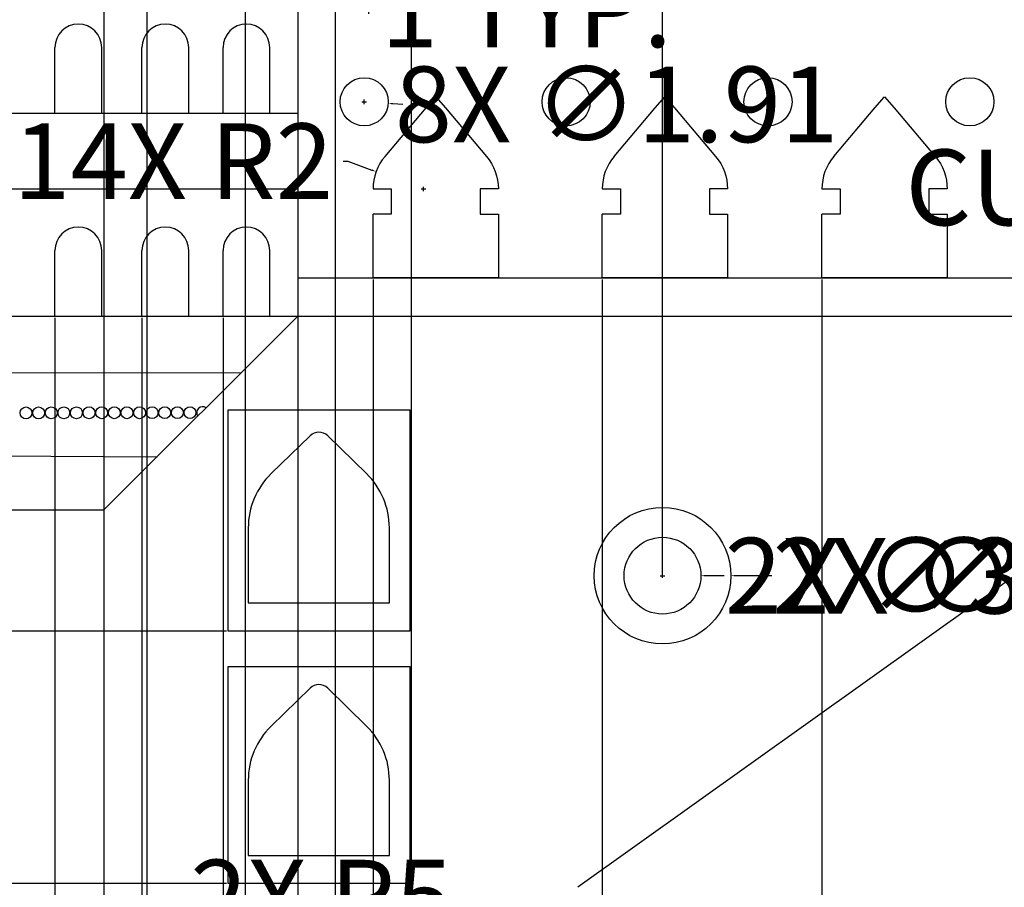
# Model space of a CAD drawing. Units: inches. Extents: x 168 to 318, y 152 to 314.
# Tile 3 of 7: x 201 to 240, y 183 to 218. Entities that reach past the tile are written whole.
import ezdxf

# ---------------------------------------------------------------- set-up
doc = ezdxf.new("R2010")
doc.units = ezdxf.units.IN
doc.header["$MEASUREMENT"] = 0
doc.layers.add('A-ANNO-DIMS', color=2, linetype='Continuous', lineweight=18)
doc.layers.add('A-ELEV', color=7, linetype='Continuous', lineweight=25)
doc.styles.get("Standard").update_dxf_attribs({"font": 'arial.ttf'})
doc.dimstyles.get("Standard").update_dxf_attribs({"dimtxt": 3, "dimasz": 0.18, "dimexe": 0.18, "dimexo": 0.0625, "dimgap": 0.09, "dimtad": 0, "dimtih": 1, "dimtoh": 1, "dimdec": 1, "dimzin": 0, "dimdsep": 46, "dimlunit": 3, "dimtxsty": 'Standard', "dimcen": 0.09, "dimadec": 0, "dimazin": 0, "dimtfac": 1, "dimtdec": 1, "dimtofl": 0, "dimtmove": 0, "dimatfit": 3, "dimfxl": 1, "dimtolj": 1, "dimtzin": 0, "dimarcsym": 0})

# ---------------------------------------------------------------- blocks, each defined once
blk = doc.blocks.new('ARCH-BALCONY-SM')
for p, q in [((0, 0), (0, 2.603)), ((1.853, 0), (1.853, 2.603))]:
    blk.add_line(p, q)
blk.add_arc((0.926, 2.603), 0.926, 0, 180)
blk = doc.blocks.new('ARCH-CUSPED-PANEL')
for p, q in [((2.1, 6.738), (2.482, 7.168)), ((2.482, 7.168), (2.864, 6.738)), ((0.472, 4.813), (2.1, 6.738)), ((2.864, 6.738), (4.491, 4.813)), ((0, 3.522), (0.2, 3.522)), ((0, 3.522), (0, 3.522)), ((0.2, 3.522), (0.719, 3.522)), ((0.719, 3.522), (0.719, 2.522)), ((4.764, 3.522), (4.244, 3.522)), ((4.244, 3.522), (4.244, 2.522)), ((4.964, 3.522), (4.764, 3.522)), ((0.719, 2.522), (0, 2.522)), ((4.244, 2.522), (4.964, 2.522))]:
    blk.add_line(p, q)
blk.add_lwpolyline([(4.491, 4.813, -0.177277), (4.964, 3.522)], format="xyb")
blk.add_lwpolyline([(4.964, 2.522), (4.964, 0), (0, 0), (0, 2.522)])
blk.add_arc((2, 3.522), 2, 139.7888, 180)
blk = doc.blocks.new('NICHE-ARCHED')
for p, q in [((0.908, 5.124), (2.451, 6.627)), ((3.149, 6.626), (4.687, 5.124)), ((0, 2.975), (0, 0)), ((5.592, 0), (5.592, 2.977)), ((0, 0), (5.592, 0))]:
    blk.add_line(p, q)
for centre, radius, start, end in [((2.8, 6.268), 0.5, 45.6844, 134.2257), ((3, 2.975), 3, 134.2257, 180), ((2.592, 2.977), 3, 0, 45.6844)]:
    blk.add_arc(centre, radius, start, end)
blk = doc.blocks.new('*D15')
at = {"layer": 'A-ANNO-DIMS', "color": 0, "lineweight": -2, "ltscale": 0.2, "transparency": 16777216}
for p, q in [((214.946, 220.875), (215.434, 220.875)), ((215.254, 220.875), (215.254, 221.055)), ((215.254, 221.055), (215.434, 221.055)), ((215.254, 218.586), (215.254, 220.695)), ((214.946, 218.406), (215.434, 218.406))]:
    blk.add_line(p, q, dxfattribs=at)
at = {"layer": 'A-ANNO-DIMS', "color": 0, "ltscale": 0.2, "transparency": 16777216}
for points in [[(215.224, 220.695), (215.284, 220.695), (215.254, 220.875)], [(215.224, 218.586), (215.284, 218.586), (215.254, 218.406)]]:
    blk.add_solid(points, dxfattribs=at)
at = {"layer": 'Defpoints', "color": 0, "ltscale": 0.2, "transparency": 16777216}
for p in [(214.883, 220.875), (215.254, 220.875), (214.883, 218.406)]:
    blk.add_point(p, dxfattribs=at)
at = {"layer": 'A-ANNO-DIMS', "color": 0, "ltscale": 0.2, "transparency": 16777216, "insert": (244.753, 221.055), "char_height": 3, "attachment_point": 5}
blk.add_mtext('\\A1;PENDANT ORNAMENT 2 TYP.', dxfattribs=at)
blk = doc.blocks.new('*D16')
at = {"layer": 'A-ANNO-DIMS', "color": 0, "lineweight": -2, "ltscale": 0.2, "transparency": 16777216}
for p, q in [((213.573, 218.343), (213.573, 217.855)), ((214.883, 218.343), (214.883, 217.855)), ((213.753, 218.035), (214.703, 218.035)), ((214.883, 218.035), (215.063, 218.035))]:
    blk.add_line(p, q, dxfattribs=at)
at = {"layer": 'A-ANNO-DIMS', "color": 0, "ltscale": 0.2, "transparency": 16777216}
for points in [[(213.753, 218.065), (213.753, 218.005), (213.573, 218.035)], [(214.703, 218.065), (214.703, 218.005), (214.883, 218.035)]]:
    blk.add_solid(points, dxfattribs=at)
at = {"layer": 'Defpoints', "color": 0, "ltscale": 0.2, "transparency": 16777216}
for p in [(213.573, 218.406), (214.883, 218.406), (214.883, 218.035)]:
    blk.add_point(p, dxfattribs=at)
at = {"layer": 'A-ANNO-DIMS', "color": 0, "ltscale": 0.2, "transparency": 16777216, "insert": (221.148, 218.035), "char_height": 3, "attachment_point": 5}
blk.add_mtext('\\A1;1 TYP.', dxfattribs=at)
blk = doc.blocks.new('*D23')
at = {"layer": 'A-ANNO-DIMS', "color": 0, "lineweight": -2, "ltscale": 0.2, "transparency": 16777216}
for p, q in [((261.882, 214.562), (263.075, 214.562)), ((262.895, 214.382), (262.895, 212.619)), ((262.895, 207.574), (262.895, 209.337)), ((261.882, 207.394), (263.075, 207.394))]:
    blk.add_line(p, q, dxfattribs=at)
at = {"layer": 'A-ANNO-DIMS', "color": 0, "ltscale": 0.2, "transparency": 16777216}
for points in [[(262.865, 214.382), (262.925, 214.382), (262.895, 214.562)], [(262.865, 207.574), (262.925, 207.574), (262.895, 207.394)]]:
    blk.add_solid(points, dxfattribs=at)
at = {"layer": 'Defpoints', "color": 0, "ltscale": 0.2, "transparency": 16777216}
for p in [(261.82, 214.562), (262.895, 214.562), (261.82, 207.394)]:
    blk.add_point(p, dxfattribs=at)
at = {"layer": 'A-ANNO-DIMS', "color": 0, "ltscale": 0.2, "transparency": 16777216, "insert": (262.895, 210.978), "char_height": 3, "attachment_point": 5}
blk.add_mtext('\\A1;CUSPED ARCH PANEL 7 TYP.', dxfattribs=at)
blk = doc.blocks.new('*D29')
at = {"layer": 'A-ANNO-DIMS', "color": 0, "lineweight": -2, "ltscale": 0.2, "transparency": 16777216}
for p, q in [((184.724, 242.139), (184.724, 154.215)), ((299.445, 242.139), (299.445, 154.215)), ((184.904, 154.395), (235.924, 154.395)), ((299.265, 154.395), (248.245, 154.395))]:
    blk.add_line(p, q, dxfattribs=at)
at = {"layer": 'A-ANNO-DIMS', "color": 0, "ltscale": 0.2, "transparency": 16777216}
for points in [[(184.904, 154.425), (184.904, 154.365), (184.724, 154.395)], [(299.265, 154.425), (299.265, 154.365), (299.445, 154.395)]]:
    blk.add_solid(points, dxfattribs=at)
at = {"layer": 'Defpoints', "color": 0, "ltscale": 0.2, "transparency": 16777216}
for p in [(184.724, 242.201), (299.445, 242.201), (299.445, 154.395)]:
    blk.add_point(p, dxfattribs=at)
at = {"layer": 'A-ANNO-DIMS', "color": 0, "ltscale": 0.2, "transparency": 16777216, "insert": (242.084, 154.395), "char_height": 3, "attachment_point": 5}
blk.add_mtext('\\A1;114.72', dxfattribs=at)
blk = doc.blocks.new('*D57')
at = {"layer": 'A-ANNO-DIMS', "color": 0, "lineweight": -2, "ltscale": 0.2, "transparency": 16777216}
for p, q in [((226.54, 195.647), (226.54, 312.411)), ((226.72, 312.231), (236.931, 312.231)), ((257.449, 312.231), (247.238, 312.231)), ((257.629, 195.647), (257.629, 312.411))]:
    blk.add_line(p, q, dxfattribs=at)
at = {"layer": 'A-ANNO-DIMS', "color": 0, "ltscale": 0.2, "transparency": 16777216}
for points in [[(226.72, 312.261), (226.72, 312.201), (226.54, 312.231)], [(257.449, 312.261), (257.449, 312.201), (257.629, 312.231)]]:
    blk.add_solid(points, dxfattribs=at)
at = {"layer": 'Defpoints', "color": 0, "ltscale": 0.2, "transparency": 16777216}
for p in [(257.629, 312.231), (226.54, 195.584), (257.629, 195.584)]:
    blk.add_point(p, dxfattribs=at)
at = {"layer": 'A-ANNO-DIMS', "color": 0, "ltscale": 0.2, "transparency": 16777216, "insert": (242.084, 312.231), "char_height": 3, "attachment_point": 5}
blk.add_mtext('\\A1;31.09', dxfattribs=at)
blk = doc.blocks.new('*D61')
at = {"layer": 'A-ANNO-DIMS', "color": 0, "lineweight": -2, "ltscale": 0.2, "transparency": 16777216}
for p, q in [((209.262, 183.379), (176.701, 183.379)), ((176.881, 183.199), (176.881, 179.852)), ((176.881, 173.262), (176.881, 176.609)), ((209.262, 173.082), (176.701, 173.082))]:
    blk.add_line(p, q, dxfattribs=at)
at = {"layer": 'A-ANNO-DIMS', "color": 0, "ltscale": 0.2, "transparency": 16777216}
for points in [[(176.851, 183.199), (176.911, 183.199), (176.881, 183.379)], [(176.851, 173.262), (176.911, 173.262), (176.881, 173.082)]]:
    blk.add_solid(points, dxfattribs=at)
at = {"layer": 'Defpoints', "color": 0, "ltscale": 0.2, "transparency": 16777216}
for p in [(176.881, 183.379), (209.325, 183.379), (209.325, 173.082)]:
    blk.add_point(p, dxfattribs=at)
at = {"layer": 'A-ANNO-DIMS', "color": 0, "ltscale": 0.2, "transparency": 16777216, "insert": (176.881, 178.231), "char_height": 3, "attachment_point": 5}
blk.add_mtext('\\A1;10.296', dxfattribs=at)
blk = doc.blocks.new('*D62')
at = {"layer": 'A-ANNO-DIMS', "color": 0, "lineweight": -2, "ltscale": 0.2, "transparency": 16777216}
for p, q in [((209.262, 193.388), (176.701, 193.388)), ((176.881, 193.208), (176.881, 190.005)), ((176.881, 183.559), (176.881, 186.762)), ((209.262, 183.379), (176.701, 183.379))]:
    blk.add_line(p, q, dxfattribs=at)
at = {"layer": 'A-ANNO-DIMS', "color": 0, "ltscale": 0.2, "transparency": 16777216}
for points in [[(176.851, 193.208), (176.911, 193.208), (176.881, 193.388)], [(176.851, 183.559), (176.911, 183.559), (176.881, 183.379)]]:
    blk.add_solid(points, dxfattribs=at)
at = {"layer": 'Defpoints', "color": 0, "ltscale": 0.2, "transparency": 16777216}
for p in [(176.881, 193.388), (209.325, 193.388), (209.325, 183.379)]:
    blk.add_point(p, dxfattribs=at)
at = {"layer": 'A-ANNO-DIMS', "color": 0, "ltscale": 0.2, "transparency": 16777216, "insert": (176.881, 188.383), "char_height": 3, "attachment_point": 5}
blk.add_mtext('\\A1;10.01', dxfattribs=at)
blk = doc.blocks.new('*D70')
at = {"layer": 'A-ANNO-DIMS', "color": 0, "lineweight": -2, "ltscale": 0.2, "transparency": 16777216}
for p, q in [((190.252, 205.813), (190.252, 154.215)), ((194.576, 205.813), (194.576, 154.215)), ((190.432, 154.395), (194.396, 154.395)), ((194.576, 154.395), (194.756, 154.395))]:
    blk.add_line(p, q, dxfattribs=at)
at = {"layer": 'A-ANNO-DIMS', "color": 0, "ltscale": 0.2, "transparency": 16777216}
for points in [[(190.432, 154.425), (190.432, 154.365), (190.252, 154.395)], [(194.396, 154.425), (194.396, 154.365), (194.576, 154.395)]]:
    blk.add_solid(points, dxfattribs=at)
at = {"layer": 'Defpoints', "color": 0, "ltscale": 0.2, "transparency": 16777216}
for p in [(190.252, 205.875), (194.576, 205.875), (194.576, 154.395)]:
    blk.add_point(p, dxfattribs=at)
at = {"layer": 'A-ANNO-DIMS', "color": 0, "ltscale": 0.2, "transparency": 16777216, "insert": (199.968, 154.395), "char_height": 3, "attachment_point": 5}
blk.add_mtext('\\A1;4.323', dxfattribs=at)
blk = doc.blocks.new('*D71')
at = {"layer": 'A-ANNO-DIMS', "color": 0, "lineweight": -2, "ltscale": 0.2, "transparency": 16777216}
for p, q in [((194.576, 205.813), (194.576, 154.215)), ((198.404, 205.813), (198.404, 154.215)), ((194.756, 154.395), (198.224, 154.395)), ((198.404, 154.395), (198.584, 154.395))]:
    blk.add_line(p, q, dxfattribs=at)
at = {"layer": 'A-ANNO-DIMS', "color": 0, "ltscale": 0.2, "transparency": 16777216}
for points in [[(194.756, 154.425), (194.756, 154.365), (194.576, 154.395)], [(198.224, 154.425), (198.224, 154.365), (198.404, 154.395)]]:
    blk.add_solid(points, dxfattribs=at)
at = {"layer": 'Defpoints', "color": 0, "ltscale": 0.2, "transparency": 16777216}
for p in [(194.576, 205.875), (198.404, 205.875), (198.404, 154.395)]:
    blk.add_point(p, dxfattribs=at)
at = {"layer": 'A-ANNO-DIMS', "color": 0, "ltscale": 0.2, "transparency": 16777216, "insert": (203.738, 154.395), "char_height": 3, "attachment_point": 5}
blk.add_mtext('\\A1;3.829', dxfattribs=at)
blk = doc.blocks.new('*D72')
at = {"layer": 'A-ANNO-DIMS', "color": 0, "lineweight": -2, "ltscale": 0.2, "transparency": 16777216}
for p, q in [((198.404, 205.813), (198.404, 154.215)), ((202.463, 205.813), (202.463, 154.215)), ((198.584, 154.395), (202.283, 154.395)), ((202.463, 154.395), (202.643, 154.395))]:
    blk.add_line(p, q, dxfattribs=at)
at = {"layer": 'A-ANNO-DIMS', "color": 0, "ltscale": 0.2, "transparency": 16777216}
for points in [[(198.584, 154.425), (198.584, 154.365), (198.404, 154.395)], [(202.283, 154.425), (202.283, 154.365), (202.463, 154.395)]]:
    blk.add_solid(points, dxfattribs=at)
at = {"layer": 'Defpoints', "color": 0, "ltscale": 0.2, "transparency": 16777216}
for p in [(198.404, 205.875), (202.463, 205.875), (202.463, 154.395)]:
    blk.add_point(p, dxfattribs=at)
at = {"layer": 'A-ANNO-DIMS', "color": 0, "ltscale": 0.2, "transparency": 16777216, "insert": (207.858, 154.395), "char_height": 3, "attachment_point": 5}
blk.add_mtext('\\A1;4.058', dxfattribs=at)
blk = doc.blocks.new('*D73')
at = {"layer": 'A-ANNO-DIMS', "color": 0, "lineweight": -2, "ltscale": 0.2, "transparency": 16777216}
for p, q in [((202.463, 205.813), (202.463, 154.215)), ((205.91, 205.813), (205.91, 154.215)), ((202.643, 154.395), (205.73, 154.395)), ((205.91, 154.395), (206.09, 154.395))]:
    blk.add_line(p, q, dxfattribs=at)
at = {"layer": 'A-ANNO-DIMS', "color": 0, "ltscale": 0.2, "transparency": 16777216}
for points in [[(202.643, 154.425), (202.643, 154.365), (202.463, 154.395)], [(205.73, 154.425), (205.73, 154.365), (205.91, 154.395)]]:
    blk.add_solid(points, dxfattribs=at)
at = {"layer": 'Defpoints', "color": 0, "ltscale": 0.2, "transparency": 16777216}
for p in [(202.463, 205.875), (205.91, 205.875), (205.91, 154.395)]:
    blk.add_point(p, dxfattribs=at)
at = {"layer": 'A-ANNO-DIMS', "color": 0, "ltscale": 0.2, "transparency": 16777216, "insert": (211.24, 154.395), "char_height": 3, "attachment_point": 5}
blk.add_mtext('\\A1;3.447', dxfattribs=at)
blk = doc.blocks.new('*D74')
at = {"layer": 'A-ANNO-DIMS', "color": 0, "lineweight": -2, "ltscale": 0.2, "transparency": 16777216}
for p, q in [((205.91, 205.813), (205.91, 154.215)), ((209.123, 205.813), (209.123, 154.215)), ((206.09, 154.395), (208.943, 154.395)), ((209.123, 154.395), (209.303, 154.395))]:
    blk.add_line(p, q, dxfattribs=at)
at = {"layer": 'A-ANNO-DIMS', "color": 0, "ltscale": 0.2, "transparency": 16777216}
for points in [[(206.09, 154.425), (206.09, 154.365), (205.91, 154.395)], [(208.943, 154.425), (208.943, 154.365), (209.123, 154.395)]]:
    blk.add_solid(points, dxfattribs=at)
at = {"layer": 'Defpoints', "color": 0, "ltscale": 0.2, "transparency": 16777216}
for p in [(205.91, 205.875), (209.123, 205.875), (209.123, 154.395)]:
    blk.add_point(p, dxfattribs=at)
at = {"layer": 'A-ANNO-DIMS', "color": 0, "ltscale": 0.2, "transparency": 16777216, "insert": (214.453, 154.395), "char_height": 3, "attachment_point": 5}
blk.add_mtext('\\A1;3.213', dxfattribs=at)
blk = doc.blocks.new('*D84')
at = {"layer": 'A-ANNO-DIMS', "color": 0, "lineweight": -2, "ltscale": 0.2, "transparency": 16777216}
for p, q in [((206.099, 227.876), (206.099, 154.215)), ((204.404, 227.113), (204.404, 154.215)), ((204.584, 154.395), (205.919, 154.395)), ((206.099, 154.395), (206.279, 154.395))]:
    blk.add_line(p, q, dxfattribs=at)
at = {"layer": 'A-ANNO-DIMS', "color": 0, "ltscale": 0.2, "transparency": 16777216}
for points in [[(204.584, 154.425), (204.584, 154.365), (204.404, 154.395)], [(205.919, 154.425), (205.919, 154.365), (206.099, 154.395)]]:
    blk.add_solid(points, dxfattribs=at)
at = {"layer": 'Defpoints', "color": 0, "ltscale": 0.2, "transparency": 16777216}
for p in [(206.099, 227.938), (204.404, 227.175), (206.099, 154.395)]:
    blk.add_point(p, dxfattribs=at)
at = {"layer": 'A-ANNO-DIMS', "color": 0, "ltscale": 0.2, "transparency": 16777216, "insert": (211.283, 154.395), "char_height": 3, "attachment_point": 5}
blk.add_mtext('\\A1;1.694', dxfattribs=at)
blk = doc.blocks.new('*D85')
at = {"layer": 'A-ANNO-DIMS', "color": 0, "lineweight": -2, "ltscale": 0.2, "transparency": 16777216}
for p, q in [((206.099, 227.876), (206.099, 154.215)), ((209.999, 227.876), (209.999, 154.215)), ((206.279, 154.395), (209.819, 154.395)), ((209.999, 154.395), (210.179, 154.395))]:
    blk.add_line(p, q, dxfattribs=at)
at = {"layer": 'A-ANNO-DIMS', "color": 0, "ltscale": 0.2, "transparency": 16777216}
for points in [[(206.279, 154.425), (206.279, 154.365), (206.099, 154.395)], [(209.819, 154.425), (209.819, 154.365), (209.999, 154.395)]]:
    blk.add_solid(points, dxfattribs=at)
at = {"layer": 'Defpoints', "color": 0, "ltscale": 0.2, "transparency": 16777216}
for p in [(206.099, 227.938), (209.999, 227.938), (209.999, 154.395)]:
    blk.add_point(p, dxfattribs=at)
at = {"layer": 'A-ANNO-DIMS', "color": 0, "ltscale": 0.2, "transparency": 16777216, "insert": (213.002, 154.395), "char_height": 3, "attachment_point": 5}
blk.add_mtext('\\A1;3.9', dxfattribs=at)
blk = doc.blocks.new('*D86')
at = {"layer": 'A-ANNO-DIMS', "color": 0, "lineweight": -2, "ltscale": 0.2, "transparency": 16777216}
for p, q in [((212.084, 220.813), (212.084, 154.215)), ((213.573, 220.813), (213.573, 154.215)), ((212.264, 154.395), (213.393, 154.395)), ((213.573, 154.395), (213.753, 154.395))]:
    blk.add_line(p, q, dxfattribs=at)
at = {"layer": 'A-ANNO-DIMS', "color": 0, "ltscale": 0.2, "transparency": 16777216}
for points in [[(212.264, 154.425), (212.264, 154.365), (212.084, 154.395)], [(213.393, 154.425), (213.393, 154.365), (213.573, 154.395)]]:
    blk.add_solid(points, dxfattribs=at)
at = {"layer": 'Defpoints', "color": 0, "ltscale": 0.2, "transparency": 16777216}
for p in [(212.084, 220.875), (213.573, 220.875), (213.573, 154.395)]:
    blk.add_point(p, dxfattribs=at)
at = {"layer": 'A-ANNO-DIMS', "color": 0, "ltscale": 0.2, "transparency": 16777216, "insert": (217.601, 154.395), "char_height": 3, "attachment_point": 5}
blk.add_mtext('\\A1;1.49', dxfattribs=at)
blk = doc.blocks.new('*D87')
at = {"layer": 'A-ANNO-DIMS', "color": 0, "lineweight": -2, "ltscale": 0.2, "transparency": 16777216}
for p, q in [((213.573, 220.813), (213.573, 154.215)), ((216.573, 220.813), (216.573, 154.215)), ((213.753, 154.395), (214.001, 154.395)), ((216.393, 154.395), (216.145, 154.395))]:
    blk.add_line(p, q, dxfattribs=at)
at = {"layer": 'A-ANNO-DIMS', "color": 0, "ltscale": 0.2, "transparency": 16777216}
for points in [[(213.753, 154.425), (213.753, 154.365), (213.573, 154.395)], [(216.393, 154.425), (216.393, 154.365), (216.573, 154.395)]]:
    blk.add_solid(points, dxfattribs=at)
at = {"layer": 'Defpoints', "color": 0, "ltscale": 0.2, "transparency": 16777216}
for p in [(213.573, 220.875), (216.573, 220.875), (216.573, 154.395)]:
    blk.add_point(p, dxfattribs=at)
at = {"layer": 'A-ANNO-DIMS', "color": 0, "ltscale": 0.2, "transparency": 16777216, "insert": (215.073, 154.395), "char_height": 3, "attachment_point": 5}
blk.add_mtext('\\A1;3', dxfattribs=at)
blk = doc.blocks.new('*D88')
at = {"layer": 'A-ANNO-DIMS', "color": 0, "lineweight": -2, "ltscale": 0.2, "transparency": 16777216}
for p, q in [((212.084, 207.331), (212.084, 154.215)), ((215.07, 207.331), (215.07, 154.215)), ((212.264, 154.395), (214.89, 154.395)), ((215.07, 154.395), (215.25, 154.395))]:
    blk.add_line(p, q, dxfattribs=at)
at = {"layer": 'A-ANNO-DIMS', "color": 0, "ltscale": 0.2, "transparency": 16777216}
for points in [[(212.264, 154.425), (212.264, 154.365), (212.084, 154.395)], [(214.89, 154.425), (214.89, 154.365), (215.07, 154.395)]]:
    blk.add_solid(points, dxfattribs=at)
at = {"layer": 'Defpoints', "color": 0, "ltscale": 0.2, "transparency": 16777216}
for p in [(212.084, 207.394), (215.07, 207.394), (215.07, 154.395)]:
    blk.add_point(p, dxfattribs=at)
at = {"layer": 'A-ANNO-DIMS', "color": 0, "ltscale": 0.2, "transparency": 16777216, "insert": (220.438, 154.395), "char_height": 3, "attachment_point": 5}
blk.add_mtext('\\A1;2.985', dxfattribs=at)
blk = doc.blocks.new('*D89')
at = {"layer": 'A-ANNO-DIMS', "color": 0, "lineweight": -2, "ltscale": 0.2, "transparency": 16777216}
for p, q in [((215.07, 207.331), (215.07, 154.215)), ((224.151, 207.331), (224.151, 154.215)), ((215.25, 154.395), (223.971, 154.395)), ((224.151, 154.395), (224.331, 154.395))]:
    blk.add_line(p, q, dxfattribs=at)
at = {"layer": 'A-ANNO-DIMS', "color": 0, "ltscale": 0.2, "transparency": 16777216}
for points in [[(215.25, 154.425), (215.25, 154.365), (215.07, 154.395)], [(223.971, 154.425), (223.971, 154.365), (224.151, 154.395)]]:
    blk.add_solid(points, dxfattribs=at)
at = {"layer": 'Defpoints', "color": 0, "ltscale": 0.2, "transparency": 16777216}
for p in [(215.07, 207.394), (224.151, 207.394), (224.151, 154.395)]:
    blk.add_point(p, dxfattribs=at)
at = {"layer": 'A-ANNO-DIMS', "color": 0, "ltscale": 0.2, "transparency": 16777216, "insert": (229.193, 154.395), "char_height": 3, "attachment_point": 5}
blk.add_mtext('\\A1;9.081', dxfattribs=at)
blk = doc.blocks.new('*D90')
at = {"layer": 'A-ANNO-DIMS', "color": 0, "lineweight": -2, "ltscale": 0.2, "transparency": 16777216}
for p, q in [((224.151, 207.331), (224.151, 154.215)), ((232.855, 207.331), (232.855, 154.215)), ((224.331, 154.395), (232.675, 154.395)), ((232.855, 154.395), (233.035, 154.395))]:
    blk.add_line(p, q, dxfattribs=at)
at = {"layer": 'A-ANNO-DIMS', "color": 0, "ltscale": 0.2, "transparency": 16777216}
for points in [[(224.331, 154.425), (224.331, 154.365), (224.151, 154.395)], [(232.675, 154.425), (232.675, 154.365), (232.855, 154.395)]]:
    blk.add_solid(points, dxfattribs=at)
at = {"layer": 'Defpoints', "color": 0, "ltscale": 0.2, "transparency": 16777216}
for p in [(224.151, 207.394), (232.855, 207.394), (232.855, 154.395)]:
    blk.add_point(p, dxfattribs=at)
at = {"layer": 'A-ANNO-DIMS', "color": 0, "ltscale": 0.2, "transparency": 16777216, "insert": (238.2, 154.395), "char_height": 3, "attachment_point": 5}
blk.add_mtext('\\A1;8.705', dxfattribs=at)
blk = doc.blocks.new('*D91')
at = {"layer": 'A-ANNO-DIMS', "color": 0, "lineweight": -2, "ltscale": 0.2, "transparency": 16777216}
for p, q in [((232.855, 207.331), (232.855, 154.215)), ((240.855, 207.331), (240.855, 154.215)), ((233.035, 154.395), (235.777, 154.395)), ((240.675, 154.395), (237.934, 154.395))]:
    blk.add_line(p, q, dxfattribs=at)
at = {"layer": 'A-ANNO-DIMS', "color": 0, "ltscale": 0.2, "transparency": 16777216}
for points in [[(233.035, 154.425), (233.035, 154.365), (232.855, 154.395)], [(240.675, 154.425), (240.675, 154.365), (240.855, 154.395)]]:
    blk.add_solid(points, dxfattribs=at)
at = {"layer": 'Defpoints', "color": 0, "ltscale": 0.2, "transparency": 16777216}
for p in [(232.855, 207.394), (240.855, 207.394), (240.855, 154.395)]:
    blk.add_point(p, dxfattribs=at)
at = {"layer": 'A-ANNO-DIMS', "color": 0, "ltscale": 0.2, "transparency": 16777216, "insert": (236.855, 154.395), "char_height": 3, "attachment_point": 5}
blk.add_mtext('\\A1;8', dxfattribs=at)
blk = doc.blocks.new('*D97')
at = {"layer": 'A-ANNO-DIMS', "color": 0, "lineweight": -2, "ltscale": 0.2, "transparency": 16777216}
for p, q in [((218.791, 182.822), (218.971, 182.822)), ((218.971, 182.822), (221.479, 181.532)), ((225.994, 179.161), (226.174, 179.161)), ((226.084, 179.071), (226.084, 179.251))]:
    blk.add_line(p, q, dxfattribs=at)
at = {"layer": 'A-ANNO-DIMS', "color": 0, "ltscale": 0.2, "transparency": 16777216}
blk.add_solid([(221.492, 181.558), (221.465, 181.505), (221.639, 181.449)], dxfattribs=at)
at = {"layer": 'Defpoints', "color": 0, "ltscale": 0.2, "transparency": 16777216}
for p in [(221.639, 181.449), (226.084, 179.161)]:
    blk.add_point(p, dxfattribs=at)
at = {"layer": 'A-ANNO-DIMS', "color": 0, "ltscale": 0.2, "transparency": 16777216, "insert": (213.023, 182.822), "char_height": 3, "attachment_point": 5}
blk.add_mtext('\\A1;2X R5', dxfattribs=at)
blk = doc.blocks.new('*D98')
at = {"layer": 'A-ANNO-DIMS', "color": 0, "lineweight": -2, "ltscale": 0.2, "transparency": 16777216}
for p, q in [((226.45, 195.584), (226.63, 195.584)), ((226.54, 195.494), (226.54, 195.674)), ((230.871, 195.584), (229.427, 195.584))]:
    blk.add_line(p, q, dxfattribs=at)
at = {"layer": 'A-ANNO-DIMS', "color": 0, "ltscale": 0.2, "transparency": 16777216}
blk.add_solid([(229.427, 195.614), (229.427, 195.554), (229.247, 195.584)], dxfattribs=at)
at = {"layer": 'Defpoints', "color": 0, "ltscale": 0.2, "transparency": 16777216}
for p in [(223.834, 195.585), (229.247, 195.584)]:
    blk.add_point(p, dxfattribs=at)
at = {"layer": 'A-ANNO-DIMS', "color": 0, "ltscale": 0.2, "transparency": 16777216, "insert": (240.824, 195.584), "char_height": 3, "attachment_point": 5}
blk.add_mtext('\\A1;2X ∅5.413', dxfattribs=at)
blk = doc.blocks.new('*D99')
at = {"layer": 'A-ANNO-DIMS', "color": 0, "lineweight": -2, "ltscale": 0.2, "transparency": 16777216}
for p, q in [((226.45, 195.584), (226.63, 195.584)), ((226.54, 195.494), (226.54, 195.674)), ((228.977, 195.584), (228.243, 195.584))]:
    blk.add_line(p, q, dxfattribs=at)
at = {"layer": 'A-ANNO-DIMS', "color": 0, "ltscale": 0.2, "transparency": 16777216}
blk.add_solid([(228.243, 195.614), (228.243, 195.554), (228.063, 195.584)], dxfattribs=at)
at = {"layer": 'Defpoints', "color": 0, "ltscale": 0.2, "transparency": 16777216}
for p in [(225.017, 195.585), (228.063, 195.584)]:
    blk.add_point(p, dxfattribs=at)
at = {"layer": 'A-ANNO-DIMS', "color": 0, "ltscale": 0.2, "transparency": 16777216, "insert": (238.928, 195.584), "char_height": 3, "attachment_point": 5}
blk.add_mtext('\\A1;2X ∅3.046', dxfattribs=at)
blk = doc.blocks.new('*D101')
at = {"layer": 'A-ANNO-DIMS', "color": 0, "lineweight": -2, "ltscale": 0.2, "transparency": 16777216}
for p, q in [((213.884, 212.015), (214.064, 212.015)), ((214.064, 212.015), (215.022, 211.665)), ((216.98, 210.916), (217.16, 210.916)), ((217.07, 210.826), (217.07, 211.006))]:
    blk.add_line(p, q, dxfattribs=at)
at = {"layer": 'A-ANNO-DIMS', "color": 0, "ltscale": 0.2, "transparency": 16777216}
blk.add_solid([(215.033, 211.693), (215.012, 211.637), (215.191, 211.603)], dxfattribs=at)
at = {"layer": 'Defpoints', "color": 0, "ltscale": 0.2, "transparency": 16777216}
for p in [(215.191, 211.603), (217.07, 210.916)]:
    blk.add_point(p, dxfattribs=at)
at = {"layer": 'A-ANNO-DIMS', "color": 0, "ltscale": 0.2, "transparency": 16777216, "insert": (207.144, 212.015), "char_height": 3, "attachment_point": 5}
blk.add_mtext('\\A1;14X R2', dxfattribs=at)
blk = doc.blocks.new('*D102')
at = {"layer": 'A-ANNO-DIMS', "color": 0, "lineweight": -2, "ltscale": 0.2, "transparency": 16777216}
for p, q in [((214.629, 214.372), (214.809, 214.372)), ((214.719, 214.282), (214.719, 214.462)), ((216.243, 214.27), (215.851, 214.296))]:
    blk.add_line(p, q, dxfattribs=at)
at = {"layer": 'A-ANNO-DIMS', "color": 0, "ltscale": 0.2, "transparency": 16777216}
blk.add_solid([(215.853, 214.326), (215.849, 214.266), (215.671, 214.308)], dxfattribs=at)
at = {"layer": 'Defpoints', "color": 0, "ltscale": 0.2, "transparency": 16777216}
for p in [(213.766, 214.435), (215.671, 214.308)]:
    blk.add_point(p, dxfattribs=at)
at = {"layer": 'A-ANNO-DIMS', "color": 0, "ltscale": 0.2, "transparency": 16777216, "insert": (224.717, 214.27), "char_height": 3, "attachment_point": 5}
blk.add_mtext('\\A1;8X ∅1.91', dxfattribs=at)

msp = doc.modelspace()

# ---------------------------------------------------------------- linework, layer by layer
at = {"layer": 'A-ELEV'}
for p, q in [((212.0845, 220.8755), (212.0845, 205.8755)), ((184.7244, 213.9241), (212.0845, 213.9241)), ((184.7244, 210.9241), (212.0845, 210.9241)), ((212.0845, 207.3935), (272.0845, 207.3935)), ((184.7244, 205.8755), (212.0845, 205.8755)), ((204.4044, 198.1954), (212.0845, 205.8755)), ((186.9522, 203.6477), (209.8404, 203.6314)), ((190.2158, 200.3841), (206.511, 200.302)), ((192.4044, 198.1954), (204.4044, 198.1954)), ((204.4044, 198.1954), (204.4044, 162.1954)), ((239.1785, 194.6573), (241.7939, 196.5252)), ((239.1785, 194.6573), (223.1785, 183.2299))]:
    msp.add_line(p, q, dxfattribs=at)
at = {"layer": 'A-ELEV', "ltscale": 0.2}
msp.add_line((212.0845, 205.8755), (272.0845, 205.8755), dxfattribs=at)
at = {"layer": 'A-ELEV'}
for points in [[(209.3248, 202.1566), (216.5216, 202.1566), (216.5216, 193.3878), (209.3248, 193.3878)], [(209.3248, 191.9874), (216.5216, 191.9874), (216.5216, 183.3788), (209.3248, 183.3788)]]:
    msp.add_lwpolyline(points, close=True, dxfattribs=at)
for centre, radius in [((214.7185, 214.3715), 0.9548), ((222.7185, 214.3715), 0.9548), ((230.7185, 214.3715), 0.9548), ((238.7185, 214.3715), 0.9548), ((201.3149, 202.0383), 0.2354), ((201.8149, 202.039), 0.2354), ((202.3149, 202.0397), 0.2354), ((202.8149, 202.0404), 0.2354), ((203.3149, 202.0412), 0.2354), ((203.8149, 202.0419), 0.2354), ((204.3149, 202.0426), 0.2354), ((204.8149, 202.0433), 0.2354), ((205.3149, 202.044), 0.2354), ((205.8149, 202.0447), 0.2354), ((206.3149, 202.0455), 0.2354), ((206.8149, 202.0462), 0.2354), ((207.3149, 202.0469), 0.2354), ((207.8149, 202.0476), 0.2354), ((226.5403, 195.5844), 2.7067), ((226.5403, 195.5844), 1.5229)]:
    msp.add_circle(centre, radius, dxfattribs=at)
msp.add_arc((208.3149, 202.0483), 0.2354, 54.95912, 215.04088, dxfattribs=at)

# ---------------------------------------------------------------- block references
for name, p in [('ARCH-BALCONY-SM', (202.4627, 213.9237)), ('ARCH-BALCONY-SM', (205.9096, 213.9237)), ('ARCH-BALCONY-SM', (209.1229, 213.9237)), ('ARCH-CUSPED-PANEL', (215.07, 207.394)), ('ARCH-CUSPED-PANEL', (224.151, 207.394)), ('ARCH-CUSPED-PANEL', (232.8558, 207.394)), ('ARCH-BALCONY-SM', (202.4627, 205.875)), ('ARCH-BALCONY-SM', (205.9096, 205.875)), ('ARCH-BALCONY-SM', (209.1229, 205.875)), ('NICHE-ARCHED', (210.123, 194.5059)), ('NICHE-ARCHED', (210.123, 184.4969))]:
    msp.add_blockref(name, p, dxfattribs=at)

# ---------------------------------------------------------------- dimensions: what is measured, and where the dimension line sits
at = {"layer": 'A-ANNO-DIMS', "ltscale": 0.2}
for base, p1, p2, override, picture, middle in [((257.6286, 312.2308), (226.5403, 195.5844), (257.6286, 195.5844), {"dimdec": 2, "dimlfac": 1, "dimrnd": 0, "dimzin": 0, "dimdsep": 46, "dimlunit": 2}, '*D57', (242.0845, 312.2308)), ((299.4446, 154.3954), (184.7244, 242.2013), (299.4446, 242.2013), {"dimdec": 2, "dimlfac": 1, "dimrnd": 0, "dimzin": 0, "dimdsep": 46, "dimlunit": 2}, '*D29', (242.0845, 154.3954)), ((206.0986, 154.3954), (204.4044, 227.1751), (206.0986, 227.9381), {"dimdec": 3, "dimlfac": 1, "dimrnd": 0, "dimzin": 0, "dimdsep": 46, "dimlunit": 2}, '*D84', (211.283, 154.3954)), ((209.9986, 154.3954), (206.0986, 227.9381), (209.9986, 227.9381), {"dimdec": 1, "dimlfac": 1, "dimrnd": 0, "dimzin": 0, "dimdsep": 46, "dimlunit": 2}, '*D85', (213.0015, 154.3954)), ((213.5729, 154.3954), (212.0845, 220.8755), (213.5729, 220.8755), {"dimdec": 2, "dimlfac": 1, "dimrnd": 0, "dimzin": 0, "dimdsep": 46, "dimlunit": 2}, '*D86', (217.601, 154.3954)), ((216.5729, 154.3954), (213.5729, 220.8755), (216.5729, 220.8755), {"dimdec": 0, "dimlfac": 1, "dimrnd": 0, "dimzin": 0, "dimdsep": 46, "dimlunit": 2}, '*D87', (215.0729, 154.3954)), ((215.0696, 154.3954), (212.0845, 207.3935), (215.0696, 207.3935), {"dimdec": 3, "dimlfac": 1, "dimrnd": 0, "dimzin": 0, "dimdsep": 46, "dimlunit": 2}, '*D88', (220.4382, 154.3954)), ((224.1506, 154.3954), (215.0696, 207.3935), (224.1506, 207.3935), {"dimdec": 3, "dimlfac": 1, "dimrnd": 0, "dimzin": 0, "dimdsep": 46, "dimlunit": 2}, '*D89', (229.1928, 154.3954)), ((232.8554, 154.3954), (224.1506, 207.3935), (232.8554, 207.3935), {"dimdec": 3, "dimlfac": 1, "dimrnd": 0, "dimzin": 0, "dimdsep": 46, "dimlunit": 2}, '*D90', (238.2004, 154.3954)), ((240.8554, 154.3954), (232.8554, 207.3935), (240.8554, 207.3935), {"dimdec": 0, "dimlfac": 1, "dimrnd": 0, "dimzin": 0, "dimdsep": 46, "dimlunit": 2}, '*D91', (236.8554, 154.3954)), ((194.5757, 154.3954), (190.2524, 205.8755), (194.5757, 205.8755), {"dimdec": 3, "dimlfac": 1, "dimrnd": 0, "dimzin": 0, "dimdsep": 46, "dimlunit": 2}, '*D70', (199.9678, 154.3954)), ((198.4044, 154.3954), (194.5757, 205.8755), (198.4044, 205.8755), {"dimdec": 3, "dimlfac": 1, "dimrnd": 0, "dimzin": 0, "dimdsep": 46, "dimlunit": 2}, '*D71', (203.7382, 154.3954)), ((202.4627, 154.3954), (198.4044, 205.8755), (202.4627, 205.8755), {"dimdec": 3, "dimlfac": 1, "dimrnd": 0, "dimzin": 0, "dimdsep": 46, "dimlunit": 2}, '*D72', (207.8578, 154.3954)), ((205.9096, 154.3954), (202.4627, 205.8755), (205.9096, 205.8755), {"dimdec": 3, "dimlfac": 1, "dimrnd": 0, "dimzin": 0, "dimdsep": 46, "dimlunit": 2}, '*D73', (211.2403, 154.3954)), ((209.1228, 154.3954), (205.9096, 205.8755), (209.1228, 205.8755), {"dimdec": 3, "dimlfac": 1, "dimrnd": 0, "dimzin": 0, "dimdsep": 46, "dimlunit": 2}, '*D74', (214.4535, 154.3954))]:
    dim = msp.add_linear_dim(base=base, p1=p1, p2=p2, dimstyle='Standard', override=override, dxfattribs=at)
    dim.commit()
    dim.dimension.update_dxf_attribs({"geometry": picture, "text_midpoint": middle})
for base, p1, p2, text, picture, middle in [((215.2539, 220.8755), (214.8834, 218.4056), (214.8834, 220.8755), 'PENDANT ORNAMENT <> TYP.', '*D15', (244.7534, 221.0555)), ((262.8949, 214.5622), (261.8196, 207.3935), (261.8196, 214.5622), 'CUSPED ARCH PANEL <> TYP.', '*D23', (262.8949, 210.9778))]:
    dim = msp.add_linear_dim(base=base, p1=p1, p2=p2, angle=90, text=text, dimstyle='Standard', override={"dimdec": 0, "dimrnd": 0, "dimzin": 0, "dimlunit": 2}, dxfattribs=at)
    dim.commit()
    dim.dimension.update_dxf_attribs({"geometry": picture, "text_midpoint": middle})
dim = msp.add_linear_dim(base=(214.8834, 218.0352), p1=(213.5729, 218.4056), p2=(214.8834, 218.4056), text='<> TYP.', dimstyle='Standard', override={"dimdec": 0, "dimrnd": 0, "dimzin": 0, "dimlunit": 2}, dxfattribs=at)
dim.commit()
dim.dimension.update_dxf_attribs({"geometry": '*D16', "text_midpoint": (221.1483, 218.0352)})
for p1, p2, text, override, picture, middle in [((213.7659, 214.4352), (215.6712, 214.3079), '8X <>', {"dimdec": 2, "dimlfac": 1, "dimrnd": 0, "dimzin": 0, "dimdsep": 46, "dimlunit": 2}, '*D102', (216.2428, 214.2697)), ((223.8336, 195.5848), (229.247, 195.584), '2X <>', {"dimdec": 3, "dimlfac": 1, "dimrnd": 0, "dimzin": 0, "dimdsep": 46, "dimlunit": 2}, '*D98', (230.8711, 195.5838)), ((225.0174, 195.5848), (228.0632, 195.584), '2X <>', {"dimdec": 3, "dimlfac": 1, "dimrnd": 0, "dimzin": 0, "dimdsep": 46, "dimlunit": 2}, '*D99', (228.9769, 195.5838))]:
    dim = msp.add_diameter_dim_2p(p1=p1, p2=p2, text=text, dimstyle='Standard', override=override, dxfattribs=at)
    dim.commit()
    dim.dimension.update_dxf_attribs({"geometry": picture, "text_midpoint": middle, "dimtype": 163})
for center, mpoint, text, picture, middle in [((217.0696, 210.9159), (215.1913, 211.6029), '14X <>', '*D101', (207.1435, 212.0151)), ((226.0845, 179.1611), (221.6387, 181.4492), '2X <>', '*D97', (213.0225, 182.822))]:
    dim = msp.add_radius_dim(center=center, mpoint=mpoint, text=text, dimstyle='Standard', override={"dimdec": 0, "dimlfac": 1, "dimrnd": 0, "dimzin": 0, "dimdsep": 46, "dimlunit": 2}, dxfattribs=at)
    dim.commit()
    dim.dimension.update_dxf_attribs({"geometry": picture, "text_midpoint": middle, "dimtype": 164})
for base, p1, p2, override, picture, middle in [((176.8805, 193.3878), (209.3248, 183.3788), (209.3248, 193.3878), {"dimdec": 2, "dimlfac": 1, "dimrnd": 0, "dimzin": 0, "dimdsep": 46, "dimlunit": 2}, '*D62', (176.8805, 188.3833)), ((176.8805, 183.3788), (209.3248, 173.0824), (209.3248, 183.3788), {"dimdec": 3, "dimlfac": 1, "dimrnd": 0, "dimzin": 0, "dimdsep": 46, "dimlunit": 2}, '*D61', (176.8805, 178.2306))]:
    dim = msp.add_linear_dim(base=base, p1=p1, p2=p2, angle=90, dimstyle='Standard', override=override, dxfattribs=at)
    dim.commit()
    dim.dimension.update_dxf_attribs({"geometry": picture, "text_midpoint": middle})

doc.saveas('drawing.dxf')
